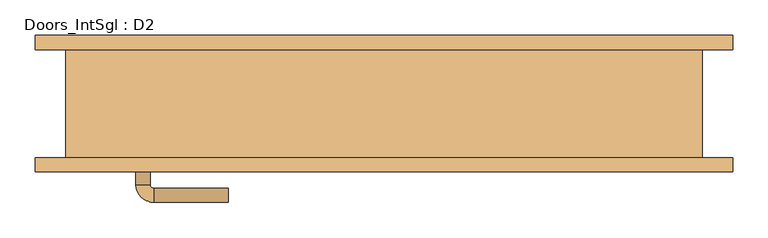
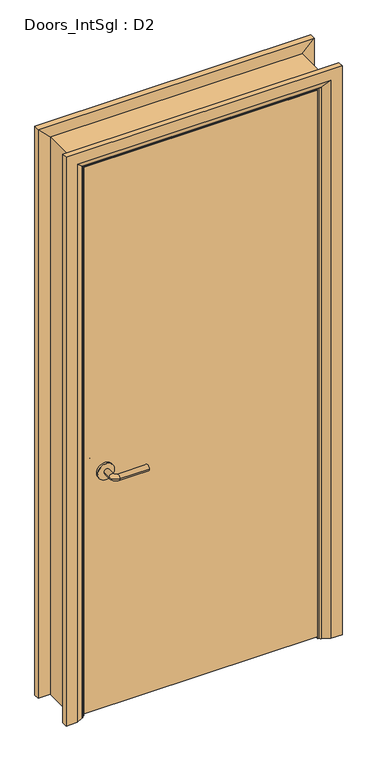
"""IFC4 building model written with IfcOpenShell, lengths in millimetres: door geometry, Doors_IntSgl : D2."""

from ifc_helpers import new_model, si_unit, point, frame, frame_2d, origin, place, context, project, spatial, polyline, circle_curve, ellipse_curve, trimmed, segment, composite_curve, outline, extrude, faceted_brep, source, transform, mapped, element, save
from ifc_brep_helpers import plane_surface, cylinder_surface, revolved_surface, advanced_brep


def doors_intsgl_d2_f2c4d474(model_context):
    return source(origin(), model_context, "Body", "SolidModel", [
        advanced_brep(
        [(-350.2, -30.2, 900.0), (-330.2, -30.2, 900.0), (-350.2, -0.2, 900.0), (-330.2, -0.2, 900.0), (-325.2, 4.8, 900.0), (-325.2, 24.8, 900.0), (-220.2, 24.8, 900.0), (-220.2, 4.8, 900.0)],
        [
            (0, 1, circle_curve(frame((-340.2, -30.2, 900.0), z_axis=(0.0, -1.0, 0.0), x_axis=(1.0, 0.0, 0.0)), 10.0)),
            (1, 0, circle_curve(frame((-340.2, -30.2, 900.0), z_axis=(0.0, -1.0, 0.0), x_axis=(1.0, 0.0, 0.0)), 10.0)),
            (0, 2),
            (2, 3, circle_curve(frame((-340.2, -0.2, 900.0), z_axis=(0.0, -1.0, 0.0), x_axis=(1.0, 0.0, 0.0)), 10.0)),
            (3, 1),
            (3, 2, circle_curve(frame((-340.2, -0.2, 900.0), z_axis=(0.0, -1.0, 0.0), x_axis=(1.0, 0.0, 0.0)), 10.0)),
            (4, 3, circle_curve(frame((-325.2, -0.2, 900.0), z_axis=(0.0, 0.0, 1.0), x_axis=(-1.0, 0.0, 0.0)), 5.0)),
            (2, 5, circle_curve(frame((-325.2, -0.2, 900.0), z_axis=(0.0, 0.0, -1.0), x_axis=(-1.0, 0.0, 0.0)), 25.0)),
            (5, 4, circle_curve(frame((-325.2, 14.8, 900.0), z_axis=(-1.0, 0.0, 0.0), x_axis=(0.0, -1.0, 0.0)), 10.0)),
            (4, 5, circle_curve(frame((-325.2, 14.8, 900.0), z_axis=(-1.0, 0.0, 0.0), x_axis=(0.0, -1.0, 0.0)), 10.0)),
            (6, 7, circle_curve(frame((-220.2, 14.8, 900.0), z_axis=(1.0, 0.0, 0.0), x_axis=(0.0, -1.0, 0.0)), 10.0)),
            (7, 6, circle_curve(frame((-220.2, 14.8, 900.0), z_axis=(1.0, 0.0, 0.0), x_axis=(0.0, -1.0, 0.0)), 10.0)),
            (5, 6),
            (7, 4),
        ],
        [
            plane_surface(frame((-340.2, -30.2, 900.0), z_axis=(0.0, -1.0, 0.0), x_axis=(0.0, 0.0, 1.0))),
            cylinder_surface(frame((-340.2, -30.2, 900.0), z_axis=(0.0, -1.0, 0.0), x_axis=(1.0, 0.0, 0.0)), 10.0),
            revolved_surface(trimmed(ellipse_curve(frame((-340.2, -0.2, 900.0), z_axis=(0.0, -1.0, 0.0), x_axis=(1.0, 0.0, 0.0)), 10.0, 10.0), [point((-350.2, -0.2, 900.0))], [point((-330.2, -0.2, 900.0))], True, "CARTESIAN"), (-325.2, -0.2, 900.0), (0.0, 0.0, -1.0)),
            revolved_surface(trimmed(ellipse_curve(frame((-340.2, -0.2, 900.0), z_axis=(0.0, -1.0, 0.0), x_axis=(1.0, 0.0, 0.0)), 10.0, 10.0), [point((-330.2, -0.2, 900.0))], [point((-350.2, -0.2, 900.0))], True, "CARTESIAN"), (-325.2, -0.2, 900.0), (0.0, 0.0, -1.0)),
            plane_surface(frame((-220.2, 14.8, 900.0), z_axis=(1.0, 0.0, 0.0), x_axis=(0.0, 0.0, 1.0))),
            cylinder_surface(frame((-325.2, 14.8, 900.0), z_axis=(-1.0, 0.0, 0.0), x_axis=(0.0, -1.0, 0.0)), 10.0),
        ],
        [
            (0, [[1, 2]]),
            (1, [[-1, 3, 4, 5]]),
            (1, [[-2, -5, 6, -3]]),
            (2, [[7, -4, 8, 9]]),
            (3, [[-8, -6, -7, 10]]),
            (4, [[11, 12]]),
            (5, [[-9, 13, -12, 14]]),
            (5, [[-10, -14, -11, -13]]),
        ],
    ),
        extrude(outline(composite_curve([segment(trimmed(circle_curve(frame_2d((900.0, -342.7)), 30.0), [point((900.0, -372.7))], [point((900.0, -312.7))], False, "CARTESIAN"), True, "CONTINUOUS"), segment(trimmed(circle_curve(frame_2d((900.0, -342.7)), 30.0), [point((900.0, -312.7))], [point((900.0, -372.7))], False, "CARTESIAN"), True, "CONTINUOUS")], self_intersect=False)), frame((0.0, -38.2, 0.0), z_axis=(0.0, 1.0, 0.0), x_axis=(0.0, 0.0, 1.0)), (0.0, 0.0, 1.0), 8.0),
        advanced_brep(
        [(-350.2, -84.2, 900.0), (-330.2, -84.2, 900.0), (-330.2, -114.2, 900.0), (-350.2, -114.2, 900.0), (-325.2, -119.2, 900.0), (-325.2, -139.2, 900.0), (-220.2, -139.2, 900.0), (-220.2, -119.2, 900.0)],
        [
            (0, 1, circle_curve(frame((-340.2, -84.2, 900.0), z_axis=(0.0, 1.0, 0.0), x_axis=(1.0, 0.0, 0.0)), 10.0)),
            (1, 0, circle_curve(frame((-340.2, -84.2, 900.0), z_axis=(0.0, 1.0, 0.0), x_axis=(1.0, 0.0, 0.0)), 10.0)),
            (1, 2),
            (2, 3, circle_curve(frame((-340.2, -114.2, 900.0), z_axis=(0.0, 1.0, 0.0), x_axis=(1.0, 0.0, 0.0)), 10.0)),
            (3, 0),
            (3, 2, circle_curve(frame((-340.2, -114.2, 900.0), z_axis=(0.0, 1.0, 0.0), x_axis=(1.0, 0.0, 0.0)), 10.0)),
            (4, 5, circle_curve(frame((-325.2, -129.2, 900.0), z_axis=(-1.0, 0.0, 0.0), x_axis=(0.0, 1.0, 0.0)), 10.0)),
            (5, 3, circle_curve(frame((-325.2, -114.2, 900.0), z_axis=(0.0, 0.0, -1.0), x_axis=(-1.0, 0.0, 0.0)), 25.0)),
            (2, 4, circle_curve(frame((-325.2, -114.2, 900.0), z_axis=(0.0, 0.0, 1.0), x_axis=(-1.0, 0.0, 0.0)), 5.0)),
            (5, 4, circle_curve(frame((-325.2, -129.2, 900.0), z_axis=(-1.0, 0.0, 0.0), x_axis=(0.0, 1.0, 0.0)), 10.0)),
            (6, 7, circle_curve(frame((-220.2, -129.2, 900.0), z_axis=(1.0, 0.0, 0.0), x_axis=(0.0, 1.0, 0.0)), 10.0)),
            (7, 6, circle_curve(frame((-220.2, -129.2, 900.0), z_axis=(1.0, 0.0, 0.0), x_axis=(0.0, 1.0, 0.0)), 10.0)),
            (4, 7),
            (6, 5),
        ],
        [
            plane_surface(frame((-340.2, -84.2, 900.0), z_axis=(0.0, 1.0, 0.0), x_axis=(0.0, 0.0, 1.0))),
            cylinder_surface(frame((-340.2, -84.2, 900.0), z_axis=(0.0, 1.0, 0.0), x_axis=(1.0, 0.0, 0.0)), 10.0),
            revolved_surface(trimmed(ellipse_curve(frame((-340.2, -114.2, 900.0), z_axis=(0.0, -1.0, 0.0), x_axis=(1.0, 0.0, 0.0)), 10.0, 10.0), [point((-350.2, -114.2, 900.0))], [point((-330.2, -114.2, 900.0))], True, "CARTESIAN"), (-325.2, -114.2, 900.0), (0.0, 0.0, -1.0)),
            revolved_surface(trimmed(ellipse_curve(frame((-340.2, -114.2, 900.0), z_axis=(0.0, -1.0, 0.0), x_axis=(1.0, 0.0, 0.0)), 10.0, 10.0), [point((-330.2, -114.2, 900.0))], [point((-350.2, -114.2, 900.0))], True, "CARTESIAN"), (-325.2, -114.2, 900.0), (0.0, 0.0, -1.0)),
            plane_surface(frame((-220.2, -129.2, 900.0), z_axis=(1.0, 0.0, 0.0), x_axis=(0.0, 0.0, 1.0))),
            cylinder_surface(frame((-325.2, -129.2, 900.0), z_axis=(-1.0, 0.0, 0.0), x_axis=(0.0, 1.0, 0.0)), 10.0),
        ],
        [
            (0, [[1, 2]]),
            (1, [[3, 4, 5, -2]]),
            (1, [[-5, 6, -3, -1]]),
            (2, [[7, 8, -4, 9]]),
            (3, [[10, -9, -6, -8]]),
            (4, [[11, 12]]),
            (5, [[13, -11, 14, -7]]),
            (5, [[-14, -12, -13, -10]]),
        ],
    ),
        extrude(outline(composite_curve([segment(trimmed(circle_curve(frame_2d((900.0, -342.7)), 30.0), [point((900.0, -372.7))], [point((900.0, -312.7))], False, "CARTESIAN"), True, "CONTINUOUS"), segment(trimmed(circle_curve(frame_2d((900.0, -342.7)), 30.0), [point((900.0, -312.7))], [point((900.0, -372.7))], False, "CARTESIAN"), True, "CONTINUOUS")], self_intersect=False)), frame((0.0, -84.2, 0.0), z_axis=(0.0, 1.0, 0.0), x_axis=(0.0, 0.0, 1.0)), (0.0, 0.0, 1.0), 8.0),
        extrude(outline(polyline([(415.2, -38.2), (415.2, -76.2), (-415.2, -76.2), (-415.2, -38.2), (415.2, -38.2)])), frame((0.0, 0.0, 8.0), z_axis=(0.0, 0.0, 1.0), x_axis=(1.0, 0.0, 0.0)), (0.0, 0.0, 1.0), 2060.0),
        advanced_brep(
        [(492.2, -96.2, 0.0), (452.2, -96.2, 0.0), (426.2, -82.2, 0.0), (422.2, -76.2, 0.0), (492.2, -76.2, 0.0), (492.2, -76.2, 2145.0), (492.2, -96.2, 2145.0), (422.2, -76.2, 2075.0), (-422.2, -76.2, 2075.0), (-422.2, -76.2, 0.0), (-492.2, -76.2, 0.0), (-492.2, -76.2, 2145.0), (426.2, -82.2, 2079.0), (452.2, -96.2, 2105.0), (-492.2, -96.2, 2145.0), (-492.2, -96.2, 0.0), (-452.2, -96.2, 0.0), (-452.2, -96.2, 2105.0), (-426.2, -82.2, 0.0), (-426.2, -82.2, 2079.0)],
        [
            (0, 1),
            (1, 2),
            (2, 3, circle_curve(frame((430.2, -75.2, 0.0), z_axis=(0.0, 0.0, -1.0), x_axis=(1.0, 0.0, 0.0)), 8.0622577)),
            (3, 4),
            (4, 0),
            (4, 5),
            (5, 6),
            (6, 0),
            (3, 7),
            (7, 8),
            (8, 9),
            (9, 10),
            (10, 11),
            (11, 5),
            (2, 12),
            (12, 7, ellipse_curve(frame((430.2, -75.2, 2083.0), z_axis=(0.7071067811865475, 0.0, -0.7071067811865475), x_axis=(-0.7071067811865474, 0.0, -0.7071067811865476)), 11.4017543, 8.0622577)),
            (1, 13),
            (13, 12),
            (6, 14),
            (14, 15),
            (15, 16),
            (16, 17),
            (17, 13),
            (10, 15),
            (14, 11),
            (9, 18, circle_curve(frame((-430.2, -75.2, 0.0), z_axis=(0.0, 0.0, -1.0), x_axis=(-1.0, 0.0, 0.0)), 8.0622577)),
            (18, 16),
            (19, 18),
            (8, 19, ellipse_curve(frame((-430.2, -75.2, 2083.0), z_axis=(-0.7071067811865475, 0.0, -0.7071067811865475), x_axis=(-0.7071067811865474, 0.0, 0.7071067811865476)), 11.4017543, 8.0622577)),
            (19, 17),
            (12, 19),
        ],
        [
            plane_surface(frame((422.2, -76.2, 0.0), z_axis=(0.0, 0.0, -1.0), x_axis=(0.0, 1.0, 0.0))),
            plane_surface(frame((492.2, -96.2, 0.0), z_axis=(1.0, 0.0, 0.0), x_axis=(0.0, 0.0, 1.0))),
            plane_surface(frame((492.2, -76.2, 0.0), z_axis=(0.0, 1.0, 0.0), x_axis=(0.0, 0.0, 1.0))),
            cylinder_surface(frame((430.2, -75.2, 0.0), z_axis=(0.0, 0.0, -1.0), x_axis=(1.0, 0.0, 0.0)), 8.0622577),
            plane_surface(frame((426.2, -82.2, 0.0), z_axis=(-0.4740998230350126, -0.880471099922178, 0.0), x_axis=(0.0, 0.0, 1.0))),
            plane_surface(frame((452.2, -96.2, 0.0), z_axis=(0.0, -1.0, 0.0), x_axis=(0.0, 0.0, 1.0))),
            plane_surface(frame((-492.2, -96.2, 2145.0), z_axis=(-1.0, 0.0, 0.0), x_axis=(0.0, 0.0, -1.0))),
            plane_surface(frame((-422.2, -76.2, 0.0), z_axis=(0.0, 0.0, -1.0), x_axis=(0.0, 1.0, 0.0))),
            cylinder_surface(frame((-430.2, -75.2, 2075.0), z_axis=(0.0, 0.0, 1.0), x_axis=(-1.0, 0.0, 0.0)), 8.0622577),
            plane_surface(frame((-426.2, -82.2, 2079.0), z_axis=(0.47409982303501824, -0.8804710999221749, 0.0), x_axis=(0.0, 0.0, -1.0))),
            plane_surface(frame((492.2, -96.2, 2145.0), z_axis=(0.0, 0.0, 1.0), x_axis=(-1.0, 0.0, 0.0))),
            cylinder_surface(frame((422.2, -75.2, 2083.0), z_axis=(1.0, 0.0, 0.0), x_axis=(0.0, 0.0, 1.0)), 8.0622577),
            plane_surface(frame((426.2, -82.2, 2079.0), z_axis=(0.0, -0.8804710999221764, -0.4740998230350154), x_axis=(-1.0, 0.0, 0.0))),
        ],
        [
            (0, [[1, 2, 3, 4, 5]]),
            (1, [[6, 7, 8, -5]]),
            (2, [[9, 10, 11, 12, 13, 14, -6, -4]]),
            (3, [[15, 16, -9, -3]]),
            (4, [[17, 18, -15, -2]]),
            (5, [[-8, 19, 20, 21, 22, 23, -17, -1]]),
            (6, [[-13, 24, -20, 25]]),
            (7, [[-24, -12, 26, 27, -21]]),
            (8, [[28, -26, -11, 29]]),
            (9, [[-22, -27, -28, 30]]),
            (10, [[-14, -25, -19, -7]]),
            (11, [[31, -29, -10, -16]]),
            (12, [[-23, -30, -31, -18]]),
        ],
    ),
        extrude(outline(polyline([(0.0, -398.2), (2051.0, -398.2), (2051.0, 398.2), (0.0, 398.2), (0.0, 417.2), (2070.0, 417.2), (2070.0, -417.2), (0.0, -417.2), (0.0, -398.2)])), frame((0.0, -36.2, 0.0), z_axis=(0.0, 1.0, 0.0), x_axis=(0.0, 0.0, 1.0)), (0.0, 0.0, 1.0), 32.0),
        advanced_brep(
        [(-492.2, 96.2, 0.0), (-452.2, 96.2, 0.0), (-426.2, 82.2, 0.0), (-422.2, 76.2, 0.0), (-492.2, 76.2, 0.0), (-492.2, 76.2, 2145.0), (-492.2, 96.2, 2145.0), (-422.2, 76.2, 2075.0), (-426.2, 82.2, 2079.0), (-452.2, 96.2, 2105.0), (492.2, 96.2, 0.0), (492.2, 76.2, 0.0), (422.2, 76.2, 0.0), (426.2, 82.2, 0.0), (452.2, 96.2, 0.0), (492.2, 96.2, 2145.0), (452.2, 96.2, 2105.0), (426.2, 82.2, 2079.0), (422.2, 76.2, 2075.0), (492.2, 76.2, 2145.0)],
        [
            (0, 1),
            (1, 2),
            (2, 3, circle_curve(frame((-430.2, 75.2, 0.0), z_axis=(0.0, 0.0, -1.0), x_axis=(-1.0, 0.0, 0.0)), 8.0622577)),
            (3, 4),
            (4, 0),
            (4, 5),
            (5, 6),
            (6, 0),
            (3, 7),
            (7, 5),
            (2, 8),
            (8, 7, ellipse_curve(frame((-430.2, 75.2, 2083.0), z_axis=(-0.7071067811865475, 0.0, -0.7071067811865475), x_axis=(0.7071067811865474, 0.0, -0.7071067811865476)), 11.4017543, 8.0622577)),
            (1, 9),
            (9, 8),
            (6, 9),
            (10, 11),
            (11, 12),
            (12, 13, circle_curve(frame((430.2, 75.2, 0.0), z_axis=(0.0, 0.0, -1.0), x_axis=(1.0, 0.0, 0.0)), 8.0622577)),
            (13, 14),
            (14, 10),
            (15, 10),
            (14, 16),
            (16, 15),
            (13, 17),
            (17, 16),
            (12, 18),
            (18, 17, ellipse_curve(frame((430.2, 75.2, 2083.0), z_axis=(0.7071067811865475, 0.0, -0.7071067811865475), x_axis=(0.7071067811865474, 0.0, 0.7071067811865476)), 11.4017543, 8.0622577)),
            (11, 19),
            (19, 18),
            (15, 19),
            (5, 19),
            (15, 6),
            (7, 18),
            (8, 17),
            (9, 16),
        ],
        [
            plane_surface(frame((-422.2, 149.0010989, 0.0), z_axis=(0.0, 0.0, -1.0), x_axis=(1.0, 0.0, 0.0))),
            plane_surface(frame((-492.2, 96.2, 0.0), z_axis=(-1.0, 0.0, 0.0), x_axis=(0.0, 0.0, 1.0))),
            plane_surface(frame((-492.2, 76.2, 0.0), z_axis=(0.0, -1.0, 0.0), x_axis=(0.0, 0.0, 1.0))),
            cylinder_surface(frame((-430.2, 75.2, 0.0), z_axis=(0.0, 0.0, -1.0), x_axis=(-1.0, 0.0, 0.0)), 8.0622577),
            plane_surface(frame((-426.2, 82.2, 0.0), z_axis=(0.4740998230350183, 0.8804710999221749, 0.0), x_axis=(0.0, 0.0, 1.0))),
            plane_surface(frame((-452.2, 96.2, 0.0), z_axis=(0.0, 1.0, 0.0), x_axis=(0.0, 0.0, 1.0))),
            plane_surface(frame((422.2, 149.0010989, 0.0), z_axis=(0.0, 0.0, -1.0), x_axis=(-1.0, 0.0, 0.0))),
            plane_surface(frame((452.2, 96.2, 2105.0), z_axis=(0.0, 1.0, 0.0), x_axis=(0.0, 0.0, -1.0))),
            plane_surface(frame((426.2, 82.2, 2079.0), z_axis=(-0.4740998230350183, 0.8804710999221749, 0.0), x_axis=(0.0, 0.0, -1.0))),
            cylinder_surface(frame((430.2, 75.2, 2075.0), z_axis=(0.0, 0.0, 1.0), x_axis=(1.0, 0.0, 0.0)), 8.0622577),
            plane_surface(frame((492.2, 76.2, 2145.0), z_axis=(0.0, -1.0, 0.0), x_axis=(0.0, 0.0, -1.0))),
            plane_surface(frame((492.2, 96.2, 2145.0), z_axis=(1.0, 0.0, 0.0), x_axis=(0.0, 0.0, -1.0))),
            plane_surface(frame((-492.2, 96.2, 2145.0), z_axis=(0.0, 0.0, 1.0), x_axis=(1.0, 0.0, 0.0))),
            plane_surface(frame((-492.2, 76.2, 2145.0), z_axis=(0.0, -1.0, 0.0), x_axis=(1.0, 0.0, 0.0))),
            cylinder_surface(frame((-422.2, 75.2, 2083.0), z_axis=(-1.0, 0.0, 0.0), x_axis=(0.0, 0.0, 1.0)), 8.0622577),
            plane_surface(frame((-426.2, 82.2, 2079.0), z_axis=(0.0, 0.8804710999221749, -0.4740998230350183), x_axis=(1.0, 0.0, 0.0))),
            plane_surface(frame((-452.2, 96.2, 2105.0), z_axis=(0.0, 1.0, 0.0), x_axis=(1.0, 0.0, 0.0))),
        ],
        [
            (0, [[1, 2, 3, 4, 5]]),
            (1, [[6, 7, 8, -5]]),
            (2, [[9, 10, -6, -4]]),
            (3, [[11, 12, -9, -3]]),
            (4, [[13, 14, -11, -2]]),
            (5, [[-8, 15, -13, -1]]),
            (6, [[16, 17, 18, 19, 20]]),
            (7, [[21, -20, 22, 23]]),
            (8, [[-22, -19, 24, 25]]),
            (9, [[-24, -18, 26, 27]]),
            (10, [[-26, -17, 28, 29]]),
            (11, [[-28, -16, -21, 30]]),
            (12, [[31, -30, 32, -7]]),
            (13, [[33, -29, -31, -10]]),
            (14, [[34, -27, -33, -12]]),
            (15, [[35, -25, -34, -14]]),
            (16, [[-32, -23, -35, -15]]),
        ],
    ),
        faceted_brep([(-417.2, -76.2, 0.0), (-449.2, -76.2, 0.0), (-449.2, 76.2, 0.0), (-417.2, 76.2, 0.0), (-417.2, 76.2, 2070.0), (-417.2, -76.2, 2070.0), (-449.2, 76.2, 2102.0), (-449.2, -76.2, 2102.0), (417.2, -76.2, 0.0), (417.2, 76.2, 0.0), (449.2, 76.2, 0.0), (449.2, -76.2, 0.0), (417.2, -76.2, 2070.0), (449.2, -76.2, 2102.0), (449.2, 76.2, 2102.0), (417.2, 76.2, 2070.0)], [[[0, 1, 2, 3]], [[3, 4, 5, 0]], [[2, 6, 4, 3]], [[1, 7, 6, 2]], [[0, 5, 7, 1]], [[8, 9, 10, 11]], [[12, 8, 11, 13]], [[13, 11, 10, 14]], [[14, 10, 9, 15]], [[15, 9, 8, 12]], [[4, 15, 12, 5]], [[6, 14, 15, 4]], [[7, 13, 14, 6]], [[5, 12, 13, 7]]]),
    ])


if __name__ == "__main__":
    model = new_model("IFC4")
    model_context = context("Model", 3, world=origin())
    ifc_project = project(units=[si_unit("LENGTHUNIT", "METRE", prefix="MILLI")], contexts=[model_context])
    site = spatial("IfcSite", under=ifc_project)
    building = spatial("IfcBuilding", under=site)
    placement = place(None, origin())
    doors_intsgl_d2_shape = doors_intsgl_d2_f2c4d474(model_context)
    element("IfcDoor", 1, ObjectType="Doors_IntSgl : D2", at=placement, inside=building, context=model_context, shape_type="MappedRepresentation", body=[
        mapped(doors_intsgl_d2_shape, transform((0.0, 0.0, 0.0), x_axis=(1.0, 0.0, 0.0), y_axis=(0.0, 1.0, 0.0), z_axis=(0.0, 0.0, 1.0))),
    ])
    save(model, "model.ifc")

# Revit data of these elements
# Type "Doors_IntSgl : D2"
#   Type Mark = "47"
#   Type Comments = "Internal Single"
#   Operation = "SingleSwingRight"
#   Manufacturer = "Revit"
#   Keynote = "L20"
#   Description = "Internal Single Door"
#   Analytic Construction = "Metal"
#   UnderCut = 0.026247 ft
#   Tolerance = 0.006562 ft
#   Thickness = 0.124672 ft
#   Thermal Resistance (R) = 0.270117 (m²·K)/W
#   Structural Tolerance = 0.026247 ft
#   StopDepth = 0.104987 ft
#   Stop Thickness = 0.062336 ft
#   Rough Width = 3.0 ft
#   Rough Height = 6.922572 ft
#   Height to Top Lock Rail = 3.28084 ft
#   Heat Transfer Coefficient (U) = 3.7021 W/(m²·K)
#   Handle Z Distance = 2.952756 ft
#   Handle X Distance = 0.246063 ft
#   Frame Thickness = 0.104987 ft
#   Door Panel Width = 2.724409 ft
#   Door Panel Thickness = 0.124672 ft
#   Door Panel Offset = 0.0 ft
#   Height = 6.922572 ft
#   Width = 3.0 ft
#   Door Panel Height = 6.75853 ft
#   Architrave Setback = 0.016404 ft
#   Vis - Ironmongery = yes
#   Material Ironmongery = Door - Handle
#   Material Frame = Door - Frame/Mullion (1)
#   Material Door = Door - Panel
#   Material Architrave = Door - Architrave
#   Visual Light Transmittance = 0
#   Solar Heat Gain Coefficient = 0
#   Function = (empty or 0)
#   Wall Closure = (empty or 0)
# Element 1 (IfcDoor, "Doors_IntSgl : D2")
#   Materials on its faces: "Door - Architrave", "Door - Handle", "Door - Frame/Mullion (1)", "Door - Panel"
# Materials
#   "Door - Handle": colour RGB 0 0 0, transparency 0, Keynote = "P21", Cost = 0
#   "Door - Frame/Mullion (1)": class "Wood", colour RGB 212 179 113, transparency 0, Keynote = "L20", Cost = 0
#   "Door - Panel": class "Wood", colour RGB 210 159 95, transparency 0, Keynote = "L20", Cost = 0
#   "Door - Architrave": class "Wood", colour RGB 154 90 5, transparency 0, Keynote = "P20", Cost = 0
